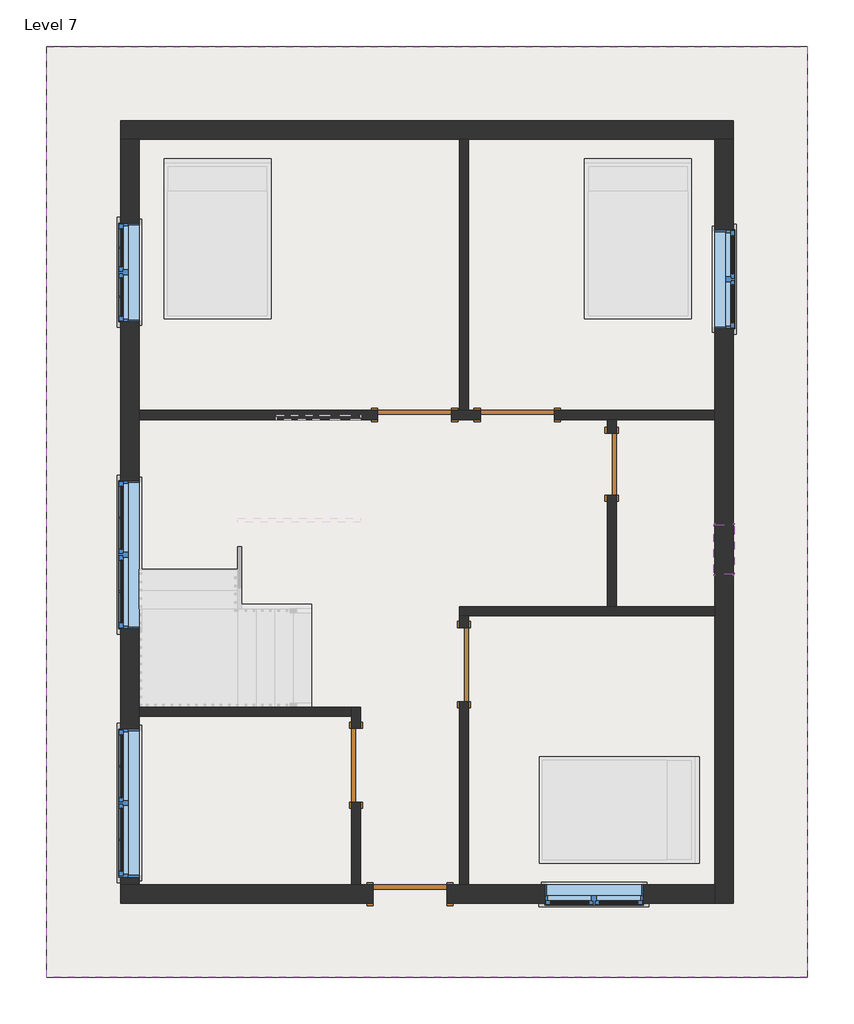
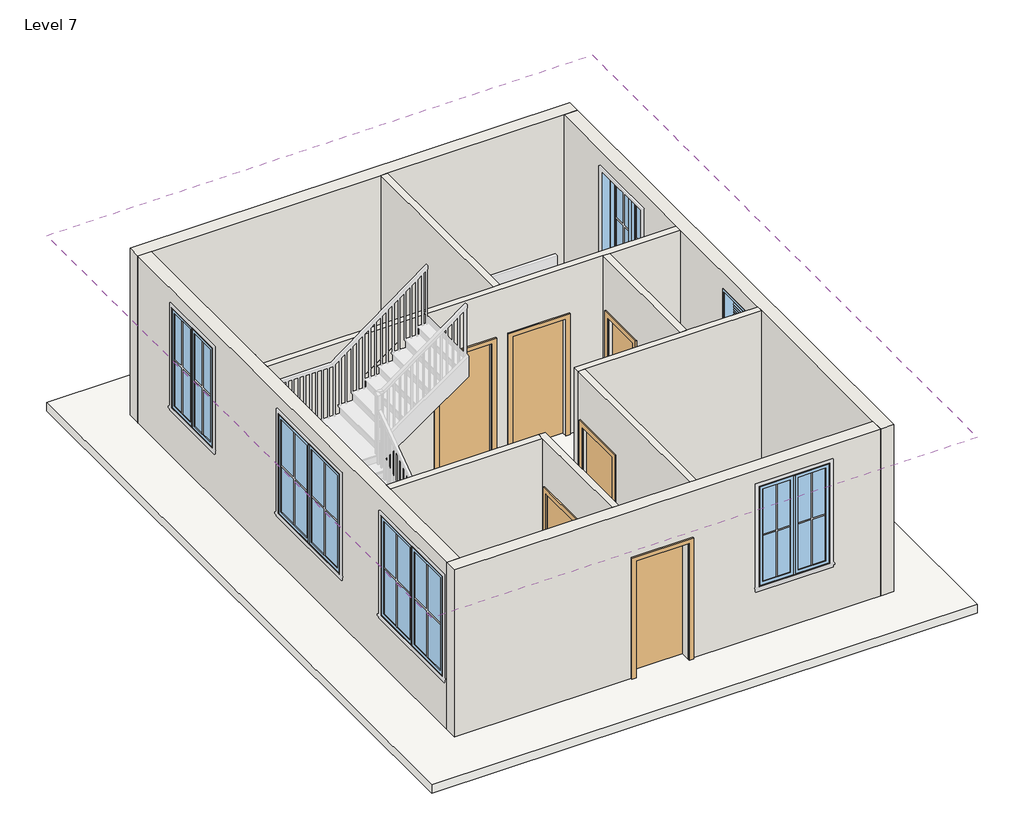
# One storey, part 1 of 3: 11 walls, 6 doors, 6 windows, 2 roofs.
"""IFC4 building model written with IfcOpenShell, lengths in millimetres."""

from ifc_helpers import new_model, si_unit, frame, origin, place, context, project, spatial, polyline, outline, extrude, faceted_brep, transform, mapped, element, save
from components import door_f2b275c1, single_flush_door_3_e5f9f3c4, single_flush_door_3_305aa2a5, single_flush_door_3_a90ba1ad, window_casement_double_win_4_6ca1769e, window_casement_double_win_6_ce442eab, window_f2d8fef0

model = new_model("IFC4")

# Units and contexts
model_context = context("Model", 3, world=origin())
ifc_project = project(units=[si_unit("LENGTHUNIT", "METRE", prefix="MILLI")], contexts=[model_context])

# Site, building, storey
site = spatial("IfcSite", under=ifc_project)
building = spatial("IfcBuilding", under=site)
storey = spatial("IfcBuildingStorey", under=building, Name="Level 7", Elevation=19050.0)

# Doors
placement = place(None, origin())
door_shape = door_f2b275c1(model_context)
element("IfcDoor", 1, ObjectType="Single-Flush : 2'6\"", at=placement, inside=storey, context=model_context, shape_type="MappedRepresentation", body=[
    mapped(door_shape, transform((1031.6394609, 262.5126239, 19050.0), x_axis=(0.0, 1.0, 0.0), y_axis=(-1.0, 0.0, 0.0), z_axis=(0.0, 0.0, 1.0))),
])
single_flush_door_3_shape = single_flush_door_3_e5f9f3c4(model_context)
element("IfcDoor", 2, ObjectType="Single-Flush : door 3'", at=placement, inside=storey, context=model_context, shape_type="MappedRepresentation", body=[
    mapped(single_flush_door_3_shape, transform((-1406.7605391, 872.1126239, 19050.0), x_axis=(1.0, 0.0, 0.0), y_axis=(0.0, 1.0, 0.0), z_axis=(0.0, 0.0, 1.0))),
])
element("IfcDoor", 3, ObjectType="Single-Flush : door 3'", at=placement, inside=storey, context=model_context, shape_type="MappedRepresentation", body=[
    mapped(single_flush_door_3_shape, transform((-2130.6605391, -3458.5873761, 19050.0), x_axis=(0.0, 1.0, 0.0), y_axis=(-1.0, 0.0, 0.0), z_axis=(0.0, 0.0, 1.0))),
])
single_flush_door_3_2_shape = single_flush_door_3_305aa2a5(model_context)
element("IfcDoor", 4, ObjectType="Single-Flush : door 3'", at=placement, inside=storey, context=model_context, shape_type="MappedRepresentation", body=[
    mapped(single_flush_door_3_2_shape, transform((-136.7605391, 872.1126239, 19050.0), x_axis=(-1.0, 0.0, 0.0), y_axis=(0.0, -1.0, 0.0), z_axis=(0.0, 0.0, 1.0))),
])
element("IfcDoor", 5, ObjectType="Single-Flush : door 3'", at=placement, inside=storey, context=model_context, shape_type="MappedRepresentation", body=[
    mapped(single_flush_door_3_2_shape, transform((-797.1605391, -2213.9873761, 19050.0), x_axis=(0.0, 1.0, 0.0), y_axis=(-1.0, 0.0, 0.0), z_axis=(0.0, 0.0, 1.0))),
])
single_flush_door_3_3_shape = single_flush_door_3_a90ba1ad(model_context)
element("IfcDoor", 6, ObjectType="Single-Flush : door 3'", at=placement, inside=storey, context=model_context, shape_type="MappedRepresentation", body=[
    mapped(single_flush_door_3_3_shape, transform((-1463.9105391, -5052.4373761, 19050.0), x_axis=(-1.0, 0.0, 0.0), y_axis=(0.0, -1.0, 0.0), z_axis=(0.0, 0.0, 1.0))),
])

# Roofs
element("IfcRoof", 7, ObjectType="Generic - 12\"", at=placement, inside=storey, context=model_context, shape_type="SweptSolid", body=[
    extrude(outline(polyline([(-5959.7105391, 5425.0626239), (3450.9894609, 5425.0626239), (3450.9894609, -6081.1373761), (-5959.7105391, -6081.1373761), (-5959.7105391, 5425.0626239)])), frame((0.0, 0.0, 18897.6), z_axis=(0.0, 0.0, 1.0), x_axis=(1.0, 0.0, 0.0)), (0.0, 0.0, 1.0), 152.4),
])
element("IfcRoof", 8, ObjectType="Generic - 12\"", at=placement, inside=storey, context=model_context, shape_type="SweptSolid", body=[
    extrude(outline(polyline([(-5959.7105391, 5425.0626239), (3450.9894609, 5425.0626239), (3450.9894609, -6081.1373761), (-5959.7105391, -6081.1373761), (-5959.7105391, 5425.0626239)])), frame((0.0, 0.0, 22098.0), z_axis=(0.0, 0.0, 1.0), x_axis=(1.0, 0.0, 0.0)), (0.0, 0.0, 1.0), 152.4),
])

# Walls
element("IfcWall", 9, ObjectType="WALL 4.5\"", at=placement, inside=storey, context=model_context, shape_type="SweptSolid", body=[
    extrude(outline(polyline([(-854.3105391, 929.2626239), (-854.3105391, 4282.0626239), (-740.0105391, 4282.0626239), (-740.0105391, 929.2626239), (-854.3105391, 929.2626239)])), frame((0.0, 0.0, 19050.0), z_axis=(0.0, 0.0, 1.0), x_axis=(1.0, 0.0, 0.0)), (0.0, 0.0, 1.0), 3048.0),
])
element("IfcWall", 10, ObjectType="WALL 4.5\"", at=placement, inside=storey, context=model_context, shape_type="Brep", body=[
    faceted_brep([(-949.5605391, 814.9626239, 19050.0), (-593.9605391, 814.9626239, 19050.0), (-593.9605391, 814.9626239, 21183.6), (320.4394609, 814.9626239, 21183.6), (320.4394609, 814.9626239, 19050.0), (974.4894609, 814.9626239, 19050.0), (1088.7894609, 814.9626239, 19050.0), (2307.9894609, 814.9626239, 19050.0), (2307.9894609, 814.9626239, 22098.0), (1088.7894609, 814.9626239, 22098.0), (974.4894609, 814.9626239, 22098.0), (-4816.7105391, 814.9626239, 22098.0), (-4816.7105391, 814.9626239, 19050.0), (-1863.9605391, 814.9626239, 19050.0), (-1863.9605391, 814.9626239, 21183.6), (-949.5605391, 814.9626239, 21183.6), (-593.9605391, 929.2626239, 21183.6), (-593.9605391, 929.2626239, 19050.0), (-740.0105391, 929.2626239, 19050.0), (-854.3105391, 929.2626239, 19050.0), (-949.5605391, 929.2626239, 19050.0), (-949.5605391, 929.2626239, 21183.6), (-1863.9605391, 929.2626239, 21183.6), (-1863.9605391, 929.2626239, 19050.0), (-4816.7105391, 929.2626239, 19050.0), (-4816.7105391, 929.2626239, 22098.0), (-854.3105391, 929.2626239, 22098.0), (-740.0105391, 929.2626239, 22098.0), (2307.9894609, 929.2626239, 22098.0), (2307.9894609, 929.2626239, 19050.0), (320.4394609, 929.2626239, 19050.0), (320.4394609, 929.2626239, 21183.6)], [[[0, 1, 2, 3, 4, 5, 6, 7, 8, 9, 10, 11, 12, 13, 14, 15]], [[16, 17, 18, 19, 20, 21, 22, 23, 24, 25, 26, 27, 28, 29, 30, 31]], [[13, 12, 24, 23]], [[30, 29, 7, 6, 5, 4]], [[20, 19, 18, 17, 1, 0]], [[8, 7, 29, 28]], [[12, 11, 25, 24]], [[21, 20, 0, 15]], [[22, 21, 15, 14]], [[23, 22, 14, 13]], [[2, 1, 17, 16]], [[3, 2, 16, 31]], [[4, 3, 31, 30]], [[11, 10, 9, 8, 28, 27, 26, 25]]]),
])
element("IfcWall", 11, ObjectType="WALL 4.5\"", at=placement, inside=storey, context=model_context, shape_type="SweptSolid", body=[
    extrude(outline(polyline([(814.9626239, 19050.0), (643.5126239, 19050.0), (643.5126239, 21082.0), (-118.4873761, 21082.0), (-118.4873761, 19050.0), (-1496.4373761, 19050.0), (-1496.4373761, 22098.0), (814.9626239, 22098.0), (814.9626239, 19050.0)])), frame((974.4894609, 0.0, 0.0), z_axis=(1.0, 0.0, 0.0), x_axis=(0.0, 1.0, 0.0)), (0.0, 0.0, 1.0), 114.3),
])
element("IfcWall", 12, ObjectType="WALL 4.5\"", at=placement, inside=storey, context=model_context, shape_type="Brep", body=[
    faceted_brep([(2307.9894609, -1496.4373761, 19050.0), (1088.7894609, -1496.4373761, 19050.0), (974.4894609, -1496.4373761, 19050.0), (-854.3105391, -1496.4373761, 19050.0), (-854.3105391, -1496.4373761, 22098.0), (974.4894609, -1496.4373761, 22098.0), (1088.7894609, -1496.4373761, 22098.0), (2307.9894609, -1496.4373761, 22098.0), (2307.9894609, -1610.7373761, 19050.0), (2307.9894609, -1610.7373761, 22098.0), (-740.0105391, -1610.7373761, 22098.0), (-854.3105391, -1610.7373761, 22098.0), (-854.3105391, -1610.7373761, 19050.0), (-740.0105391, -1610.7373761, 19050.0)], [[[0, 1, 2, 3, 4, 5, 6, 7]], [[8, 9, 10, 11, 12, 13]], [[3, 2, 1, 0, 8, 13, 12]], [[0, 7, 9, 8]], [[4, 3, 12, 11]], [[7, 6, 5, 4, 11, 10, 9]]]),
])
element("IfcWall", 13, ObjectType="WALL 4.5\"", at=placement, inside=storey, context=model_context, shape_type="SweptSolid", body=[
    extrude(outline(polyline([(-1610.7373761, 19050.0), (-1756.7873761, 19050.0), (-1756.7873761, 21183.6), (-2671.1873761, 21183.6), (-2671.1873761, 19050.0), (-4938.1373761, 19050.0), (-4938.1373761, 22098.0), (-1610.7373761, 22098.0), (-1610.7373761, 19050.0)])), frame((-854.3105391, 0.0, 0.0), z_axis=(1.0, 0.0, 0.0), x_axis=(0.0, 1.0, 0.0)), (0.0, 0.0, 1.0), 114.3),
])
element("IfcWall", 14, ObjectType="WALL 4.5\"", at=placement, inside=storey, context=model_context, shape_type="Brep", body=[
    faceted_brep([(-2073.5105391, -3001.3873761, 21183.6), (-2073.5105391, -3001.3873761, 19050.0), (-2073.5105391, -2741.0373761, 19050.0), (-2073.5105391, -2741.0373761, 22098.0), (-2073.5105391, -4938.1373761, 22098.0), (-2073.5105391, -4938.1373761, 19050.0), (-2073.5105391, -3915.7873761, 19050.0), (-2073.5105391, -3915.7873761, 21183.6), (-2187.8105391, -2741.0373761, 19050.0), (-2187.8105391, -2855.3373761, 19050.0), (-2187.8105391, -3001.3873761, 19050.0), (-2187.8105391, -3001.3873761, 21183.6), (-2187.8105391, -3915.7873761, 21183.6), (-2187.8105391, -3915.7873761, 19050.0), (-2187.8105391, -4938.1373761, 19050.0), (-2187.8105391, -4938.1373761, 22098.0), (-2187.8105391, -2855.3373761, 22098.0), (-2187.8105391, -2741.0373761, 22098.0)], [[[0, 1, 2, 3, 4, 5, 6, 7]], [[8, 9, 10, 11, 12, 13, 14, 15, 16, 17]], [[6, 5, 14, 13]], [[2, 1, 10, 9, 8]], [[5, 4, 15, 14]], [[3, 2, 8, 17]], [[11, 10, 1, 0]], [[12, 11, 0, 7]], [[13, 12, 7, 6]], [[4, 3, 17, 16, 15]]]),
])
element("IfcWall", 15, ObjectType="WALL 4.5\"", at=placement, inside=storey, context=model_context, shape_type="SweptSolid", body=[
    extrude(outline(polyline([(-4816.7105391, -2741.0373761), (-2187.8105391, -2741.0373761), (-2187.8105391, -2855.3373761), (-4816.7105391, -2855.3373761), (-4816.7105391, -2741.0373761)])), frame((0.0, 0.0, 19050.0), z_axis=(0.0, 0.0, 1.0), x_axis=(1.0, 0.0, 0.0)), (0.0, 0.0, 1.0), 3048.0),
])
element("IfcWall", 16, ObjectType="WALL 9\"", at=placement, inside=storey, context=model_context, shape_type="Brep", body=[
    faceted_brep([(-5045.3105391, 4282.0626239, 19050.0), (-4816.7105391, 4282.0626239, 19050.0), (-854.3105391, 4282.0626239, 19050.0), (-740.0105391, 4282.0626239, 19050.0), (2307.9894609, 4282.0626239, 19050.0), (2536.5894609, 4282.0626239, 19050.0), (2536.5894609, 4282.0626239, 22098.0), (2307.9894609, 4282.0626239, 22098.0), (-740.0105391, 4282.0626239, 22098.0), (-854.3105391, 4282.0626239, 22098.0), (-4816.7105391, 4282.0626239, 22098.0), (-5045.3105391, 4282.0626239, 22098.0), (-5045.3105391, 4510.6626239, 19050.0), (-5045.3105391, 4510.6626239, 22098.0), (2536.5894609, 4510.6626239, 22098.0), (2536.5894609, 4510.6626239, 19050.0)], [[[0, 1, 2, 3, 4, 5, 6, 7, 8, 9, 10, 11]], [[12, 13, 14, 15]], [[5, 4, 3, 2, 1, 0, 12, 15]], [[6, 5, 15, 14]], [[0, 11, 13, 12]], [[11, 10, 9, 8, 7, 6, 14, 13]]]),
])
element("IfcWall", 17, ObjectType="WALL 9\"", at=placement, inside=storey, context=model_context, shape_type="Brep", body=[
    faceted_brep([(2307.9894609, 4282.0626239, 19050.0), (2307.9894609, 929.2626239, 19050.0), (2307.9894609, 814.9626239, 19050.0), (2307.9894609, -1496.4373761, 19050.0), (2307.9894609, -1610.7373761, 19050.0), (2307.9894609, -4938.1373761, 19050.0), (2307.9894609, -5166.7373761, 19050.0), (2307.9894609, -5166.7373761, 22098.0), (2307.9894609, -4938.1373761, 22098.0), (2307.9894609, -1610.7373761, 22098.0), (2307.9894609, -1496.4373761, 22098.0), (2307.9894609, 814.9626239, 22098.0), (2307.9894609, 929.2626239, 22098.0), (2307.9894609, 4282.0626239, 22098.0), (2307.9894609, 1938.9126239, 21793.2), (2307.9894609, 1938.9126239, 19964.4), (2307.9894609, 3158.1126239, 19964.4), (2307.9894609, 3158.1126239, 21793.2), (2307.9894609, -486.7873761, 21793.2), (2307.9894609, -1096.3873761, 21793.2), (2307.9894609, -1096.3873761, 21183.6), (2307.9894609, -486.7873761, 21183.6), (2536.5894609, 4282.0626239, 19050.0), (2536.5894609, 4282.0626239, 22098.0), (2536.5894609, -5166.7373761, 22098.0), (2536.5894609, -5166.7373761, 19050.0), (2536.5894609, 1938.9126239, 21793.2), (2536.5894609, 3158.1126239, 21793.2), (2536.5894609, 3158.1126239, 19964.4), (2536.5894609, 1938.9126239, 19964.4), (2536.5894609, -486.7873761, 21793.2), (2536.5894609, -486.7873761, 21183.6), (2536.5894609, -1096.3873761, 21183.6), (2536.5894609, -1096.3873761, 21793.2)], [[[0, 1, 2, 3, 4, 5, 6, 7, 8, 9, 10, 11, 12, 13], [14, 15, 16, 17], [18, 19, 20, 21]], [[22, 23, 24, 25], [26, 27, 28, 29], [30, 31, 32, 33]], [[6, 5, 4, 3, 2, 1, 0, 22, 25]], [[0, 13, 23, 22]], [[7, 6, 25, 24]], [[15, 14, 26, 29]], [[16, 15, 29, 28]], [[17, 16, 28, 27]], [[14, 17, 27, 26]], [[31, 30, 18, 21]], [[32, 31, 21, 20]], [[33, 32, 20, 19]], [[30, 33, 19, 18]], [[13, 12, 11, 10, 9, 8, 7, 24, 23]]]),
])
element("IfcWall", 18, ObjectType="WALL 9\"", at=placement, inside=storey, context=model_context, shape_type="Brep", body=[
    faceted_brep([(-1921.1105391, -4938.1373761, 21183.6), (-1921.1105391, -4938.1373761, 19050.0), (-2073.5105391, -4938.1373761, 19050.0), (-2187.8105391, -4938.1373761, 19050.0), (-4816.7105391, -4938.1373761, 19050.0), (-5045.3105391, -4938.1373761, 19050.0), (-5045.3105391, -4938.1373761, 22098.0), (-4816.7105391, -4938.1373761, 22098.0), (-2187.8105391, -4938.1373761, 22098.0), (-2073.5105391, -4938.1373761, 22098.0), (-854.3105391, -4938.1373761, 22098.0), (-740.0105391, -4938.1373761, 22098.0), (2307.9894609, -4938.1373761, 22098.0), (2307.9894609, -4938.1373761, 19050.0), (-740.0105391, -4938.1373761, 19050.0), (-854.3105391, -4938.1373761, 19050.0), (-1006.7105391, -4938.1373761, 19050.0), (-1006.7105391, -4938.1373761, 21183.6), (202.9644609, -4938.1373761, 21793.2), (202.9644609, -4938.1373761, 19964.4), (1422.1644609, -4938.1373761, 19964.4), (1422.1644609, -4938.1373761, 21793.2), (-5045.3105391, -5166.7373761, 19050.0), (-1921.1105391, -5166.7373761, 19050.0), (-1921.1105391, -5166.7373761, 21183.6), (-1006.7105391, -5166.7373761, 21183.6), (-1006.7105391, -5166.7373761, 19050.0), (2307.9894609, -5166.7373761, 19050.0), (2307.9894609, -5166.7373761, 22098.0), (-5045.3105391, -5166.7373761, 22098.0), (202.9644609, -5166.7373761, 21793.2), (1422.1644609, -5166.7373761, 21793.2), (1422.1644609, -5166.7373761, 19964.4), (202.9644609, -5166.7373761, 19964.4)], [[[0, 1, 2, 3, 4, 5, 6, 7, 8, 9, 10, 11, 12, 13, 14, 15, 16, 17], [18, 19, 20, 21]], [[22, 23, 24, 25, 26, 27, 28, 29], [30, 31, 32, 33]], [[5, 4, 3, 2, 1, 23, 22]], [[16, 15, 14, 13, 27, 26]], [[13, 12, 28, 27]], [[6, 5, 22, 29]], [[19, 18, 30, 33]], [[20, 19, 33, 32]], [[21, 20, 32, 31]], [[18, 21, 31, 30]], [[24, 23, 1, 0]], [[25, 24, 0, 17]], [[26, 25, 17, 16]], [[12, 11, 10, 9, 8, 7, 6, 29, 28]]]),
])
element("IfcWall", 19, ObjectType="WALL 9\"", at=placement, inside=storey, context=model_context, shape_type="Brep", body=[
    faceted_brep([(-4816.7105391, -4938.1373761, 19050.0), (-4816.7105391, -2855.3373761, 19050.0), (-4816.7105391, -2741.0373761, 19050.0), (-4816.7105391, 814.9626239, 19050.0), (-4816.7105391, 929.2626239, 19050.0), (-4816.7105391, 4282.0626239, 19050.0), (-4816.7105391, 4282.0626239, 22098.0), (-4816.7105391, 929.2626239, 22098.0), (-4816.7105391, 814.9626239, 22098.0), (-4816.7105391, -2741.0373761, 22098.0), (-4816.7105391, -2855.3373761, 22098.0), (-4816.7105391, -4938.1373761, 22098.0), (-4816.7105391, -3010.9123761, 21793.2), (-4816.7105391, -3010.9123761, 19964.4), (-4816.7105391, -4839.7123761, 19964.4), (-4816.7105391, -4839.7123761, 21793.2), (-4816.7105391, 59.3126239, 21793.2), (-4816.7105391, 59.3126239, 19964.4), (-4816.7105391, -1769.4873761, 19964.4), (-4816.7105391, -1769.4873761, 21793.2), (-4816.7105391, 3243.8376239, 21793.2), (-4816.7105391, 3243.8376239, 19964.4), (-4816.7105391, 2024.6376239, 19964.4), (-4816.7105391, 2024.6376239, 21793.2), (-5045.3105391, -4938.1373761, 19050.0), (-5045.3105391, -4938.1373761, 22098.0), (-5045.3105391, 4282.0626239, 22098.0), (-5045.3105391, 4282.0626239, 19050.0), (-5045.3105391, -3010.9123761, 21793.2), (-5045.3105391, -4839.7123761, 21793.2), (-5045.3105391, -4839.7123761, 19964.4), (-5045.3105391, -3010.9123761, 19964.4), (-5045.3105391, 59.3126239, 21793.2), (-5045.3105391, -1769.4873761, 21793.2), (-5045.3105391, -1769.4873761, 19964.4), (-5045.3105391, 59.3126239, 19964.4), (-5045.3105391, 3243.8376239, 21793.2), (-5045.3105391, 2024.6376239, 21793.2), (-5045.3105391, 2024.6376239, 19964.4), (-5045.3105391, 3243.8376239, 19964.4)], [[[0, 1, 2, 3, 4, 5, 6, 7, 8, 9, 10, 11], [12, 13, 14, 15], [16, 17, 18, 19], [20, 21, 22, 23]], [[24, 25, 26, 27], [28, 29, 30, 31], [32, 33, 34, 35], [36, 37, 38, 39]], [[5, 4, 3, 2, 1, 0, 24, 27]], [[6, 5, 27, 26]], [[0, 11, 25, 24]], [[13, 12, 28, 31]], [[14, 13, 31, 30]], [[15, 14, 30, 29]], [[12, 15, 29, 28]], [[17, 16, 32, 35]], [[18, 17, 35, 34]], [[19, 18, 34, 33]], [[16, 19, 33, 32]], [[21, 20, 36, 39]], [[22, 21, 39, 38]], [[23, 22, 38, 37]], [[20, 23, 37, 36]], [[11, 10, 9, 8, 7, 6, 26, 25]]]),
])

# Windows
window_casement_double_win_4_shape = window_casement_double_win_4_6ca1769e(model_context)
element("IfcWindow", 20, ObjectType="Window-Casement-Double : win 4'", at=placement, inside=storey, context=model_context, shape_type="MappedRepresentation", body=[
    mapped(window_casement_double_win_4_shape, transform((812.5644609, -5052.4373761, 19050.0), x_axis=(-1.0, 0.0, 0.0), y_axis=(0.0, -1.0, 0.0), z_axis=(0.0, 0.0, 1.0))),
])
element("IfcWindow", 21, ObjectType="Window-Casement-Double : win 4'", at=placement, inside=storey, context=model_context, shape_type="MappedRepresentation", body=[
    mapped(window_casement_double_win_4_shape, transform((2422.2894609, 2548.5126239, 19050.0), x_axis=(0.0, -1.0, 0.0), y_axis=(1.0, 0.0, 0.0), z_axis=(0.0, 0.0, 1.0))),
])
element("IfcWindow", 22, ObjectType="Window-Casement-Double : win 4'", at=placement, inside=storey, context=model_context, shape_type="MappedRepresentation", body=[
    mapped(window_casement_double_win_4_shape, transform((-4931.0105391, 2634.2376239, 19050.0), x_axis=(0.0, 1.0, 0.0), y_axis=(-1.0, 0.0, 0.0), z_axis=(0.0, 0.0, 1.0))),
])
window_casement_double_win_6_shape = window_casement_double_win_6_ce442eab(model_context)
element("IfcWindow", 23, ObjectType="Window-Casement-Double : win 6'", at=placement, inside=storey, context=model_context, shape_type="MappedRepresentation", body=[
    mapped(window_casement_double_win_6_shape, transform((-4931.0105391, -3925.3123761, 19050.0), x_axis=(0.0, 1.0, 0.0), y_axis=(-1.0, 0.0, 0.0), z_axis=(0.0, 0.0, 1.0))),
])
element("IfcWindow", 24, ObjectType="Window-Casement-Double : win 6'", at=placement, inside=storey, context=model_context, shape_type="MappedRepresentation", body=[
    mapped(window_casement_double_win_6_shape, transform((-4931.0105391, -855.0873761, 19050.0), x_axis=(0.0, 1.0, 0.0), y_axis=(-1.0, 0.0, 0.0), z_axis=(0.0, 0.0, 1.0))),
])
window_shape = window_f2d8fef0(model_context)
element("IfcWindow", 25, ObjectType="Window-Louvers : 24\" x 24\"", at=placement, inside=storey, context=model_context, shape_type="MappedRepresentation", body=[
    mapped(window_shape, transform((2428.6394609, -791.5873761, 20269.2), x_axis=(0.0, -1.0, 0.0), y_axis=(1.0, 0.0, 0.0), z_axis=(0.0, 0.0, 1.0))),
])

save(model, "model.ifc")

# Revit data of these elements
# Type "Single-Flush : 2'6\""
#   Type Mark = "9"
#   Construction Type Id = "MDOOR"
#   Assembly Code = "C1020"
#   Analytic Construction = "Metal"
#   Thickness = 0' - 2"
#   Heat Transfer Coefficient (U) = 0.651978 BTU/(h·ft²·°F)
#   Height = 6' - 8"
#   Trim Projection Ext = 0' - 1"
#   Trim Projection Int = 0' - 1"
#   Trim Width = 0' - 3"
#   Width = 2' - 6"
#   Define Thermal Properties by = 1
#   Door Material = Door - Panel
#   Frame Material = Door - Frame
#   Visual Light Transmittance = 0
#   Solar Heat Gain Coefficient = 0
#   Function = (empty or 0)
#   Wall Closure = (empty or 0)
# Type "Single-Flush : door 3'"
#   Type Mark = "8"
#   Construction Type Id = "MDOOR"
#   Assembly Code = "C1020"
#   Analytic Construction = "Metal"
#   Thickness = 0' - 2"
#   Heat Transfer Coefficient (U) = 0.651978 BTU/(h·ft²·°F)
#   Height = 7' - 0"
#   Trim Projection Ext = 0' - 1"
#   Trim Projection Int = 0' - 1"
#   Trim Width = 0' - 3"
#   Width = 3' - 0"
#   Define Thermal Properties by = 1
#   Door Material = Door - Panel
#   Frame Material = Door - Frame
#   Visual Light Transmittance = 0
#   Solar Heat Gain Coefficient = 0
#   Function = (empty or 0)
#   Wall Closure = (empty or 0)
# Type "Generic - 12\""
#   Assembly Code = "B1020"
#   Layers, outside or top first: 0' - 6" no material (function 1)
# Type "WALL 4.5\""
#   Assembly Code = "B2010"
#   Layers, outside or top first: 0' - 4 1/2" no material (function 1)
# Type "WALL 9\""
#   Assembly Code = "B2010"
#   Layers, outside or top first: 0' - 9" no material (function 1)
# Type "Window-Casement-Double : win 4'"
#   Type Mark = "19"
#   Fire Rating = "0.5h"
#   Assembly Code = "B2020100"
#   Analytic Construction = "Double glazing - domestic"
#   Frame Extension [instance default] = 0' - 0 1/4"
#   Window Inset [instance default] = 0' - 0"
#   Wall Thickness [instance default] = 0' - 6"
#   Interior Wall Closure [instance default] = 0' - 2 1/4"
#   Half Width = 2' - 0"
#   Visual Light Transmittance = 0.81
#   Thermal Resistance (R) = 1.8146 (h·ft²·°F)/BTU
#   Solar Heat Gain Coefficient = 0.76
#   Rough Width = 4' - 0 1/2"
#   Rough Height = 6' - 0 1/2"
#   Height = 6' - 0"
#   Heat Transfer Coefficient (U) = 0.5511 BTU/(h·ft²·°F)
#   Exterior Wall Closure [instance default] = 0' - 1 1/4"
#   Extension Jamb [instance default] = 0' - 2 1/4"
#   Default Sill Height = 3' - 0"
#   Width = 4' - 0"
#   Muntin Visibility = yes
#   Interior Trim Visibility [instance default] = yes
#   Exterior Trim Visibility [instance default] = yes
#   Extension Jamb Visibility [instance default] = yes
#   Interior Trim Material = Wood - Stained
#   Muntin Pattern = Muntin Pattern_2x2 : Muntin Pattern_2x2
#   Interior Trim = Trim-Window-Interior-Flat : Picture Frame
#   Interior Frame Material = Wood - Stained
#   Glass Panel Material = Glass
#   Exterior Trim Material = Clad - White
#   Exterior Trim = Trim-Window-Exterior-Flat : with Sill
#   Exterior Frame Material = Clad - White
#   Wall Closure = (empty or 0)
# Type "Window-Casement-Double : win 6'"
#   Type Mark = "18"
#   Fire Rating = "0.5h"
#   Assembly Code = "B2020100"
#   Analytic Construction = "Double glazing - domestic"
#   Frame Extension [instance default] = 0' - 0 1/4"
#   Window Inset [instance default] = 0' - 0"
#   Wall Thickness [instance default] = 0' - 6"
#   Interior Wall Closure [instance default] = 0' - 2 1/4"
#   Half Width = 3' - 0"
#   Visual Light Transmittance = 0.81
#   Thermal Resistance (R) = 1.8146 (h·ft²·°F)/BTU
#   Solar Heat Gain Coefficient = 0.76
#   Rough Width = 6' - 0 1/2"
#   Rough Height = 6' - 0 1/2"
#   Height = 6' - 0"
#   Heat Transfer Coefficient (U) = 0.5511 BTU/(h·ft²·°F)
#   Exterior Wall Closure [instance default] = 0' - 1 1/4"
#   Extension Jamb [instance default] = 0' - 2 1/4"
#   Default Sill Height = 3' - 0"
#   Width = 6' - 0"
#   Muntin Visibility = yes
#   Interior Trim Visibility [instance default] = yes
#   Exterior Trim Visibility [instance default] = yes
#   Extension Jamb Visibility [instance default] = yes
#   Interior Trim Material = Wood - Stained
#   Muntin Pattern = Muntin Pattern_2x2 : Muntin Pattern_2x2
#   Interior Trim = Trim-Window-Interior-Flat : Picture Frame
#   Interior Frame Material = Wood - Stained
#   Glass Panel Material = Glass
#   Exterior Trim Material = Clad - White
#   Exterior Trim = Trim-Window-Exterior-Flat : with Sill
#   Exterior Frame Material = Clad - White
#   Wall Closure = (empty or 0)
# Type "Window-Louvers : 24\" x 24\""
#   Type Mark = "20"
#   Construction Type Id = "GSP4R"
#   Assembly Code = "B20"
#   Analytic Construction = "1/8 in Pilkington single glazing"
#   Visual Light Transmittance = 0.9
#   Thermal Resistance (R) = 1.53941 (h·ft²·°F)/BTU
#   Solar Heat Gain Coefficient = 0.78
#   Max Height = 1' - 11.74264"
#   Height = 2' - 0"
#   Heat Transfer Coefficient (U) = 0.6496 BTU/(h·ft²·°F)
#   Blade Width [instance default] = 1' - 10 1/2"
#   Blade Vertical Thickness = 0' - 0.35355"
#   Blade Thickness = 0' - 0 1/4"
#   Blade Spacing = 0' - 1 1/2"
#   Blade Height = 0' - 1.85355"
#   Blade Depth = 0' - 3"
#   Blade Angle = 45.00°
#   Default Sill Height = 3' - 0"
#   Trim Projection_Exterior = 0' - 0 1/2"
#   Trim Projection_Interior = 0' - 0 1/2"
#   Trim Width_Exterior = 0' - 1 1/2"
#   Trim Width_Interior = 0' - 1 1/2"
#   Width = 2' - 0"
#   Max Blade Count = 12
#   Define Thermal Properties by = 1
#   Blade Count = 12
#   Frame Material = Birch
#   Louver Material = Birch
#   Trim Exterior Material = Birch
#   Trim Interior Material = Birch
#   Wall Closure = (empty or 0)
# Element 1 (IfcDoor, "Single-Flush : 2'6\"")
#   Phase Created = New Construction
#   Materials on its faces: "Door - Frame", "Door - Panel"
# Elements 2, 3, 4, 5, 6 (IfcDoor, "Single-Flush : door 3'")
#   Phase Created = New Construction
#   Materials on its faces: "Door - Frame", "Door - Panel"
# Element 7 (IfcRoof, "Generic - 12\"")
#   built-in parameter 1001705 = 62.5 (stored number, unit not read)
#   built-in parameter 1001701 = -0.5 (stored number, unit not read)
#   built-in parameter 1001710 = 33615
#   Phase Created = New Construction
#   Materials on its faces: "Wood Planks", "Wood - Stained"
# Element 8 (IfcRoof, "Generic - 12\"")
#   built-in parameter 1001705 = 73 (stored number, unit not read)
#   built-in parameter 1001701 = 10 (stored number, unit not read)
#   built-in parameter 1001710 = 33615
#   Phase Created = New Construction
#   Materials on its faces: "Wood Planks", "Wood - Stained"
# Elements 9, 10, 11, 12, 13, 14, 15 (IfcWall, "WALL 4.5\"")
#   Top Offset = 0' - 0"
#   Base Offset = 0' - 0"
#   Unconnected Height = 10' - 0"
#   wall height = 10' - 0"
#   Phase Created = New Construction
#   Base Constraint = Level 7
#   Materials on its faces: "Default Wall"
# Elements 16, 17, 18, 19 (IfcWall, "WALL 9\"")
#   Top Offset = 0' - 0"
#   Base Offset = 0' - 0"
#   Unconnected Height = 10' - 0"
#   wall height = 10' - 0"
#   Phase Created = New Construction
#   Base Constraint = Level 7
#   Materials on its faces: "Default Wall", "Door - Frame"
# Element 20 (IfcWindow, "Window-Casement-Double : win 4'")
#   Mark = "39"
#   Window Inset = 0' - 0"
#   Interior Wall Closure = 0' - 2 1/4"
#   Frame Extension = 0' - 0 1/4"
#   Exterior Wall Closure = 0' - 1 1/4"
#   Interior Trim Visibility = yes
#   Exterior Trim Visibility = yes
#   Phase Created = New Construction
#   Materials on its faces: "Wood - Stained", "Glass", "Clad - White"
# Element 21 (IfcWindow, "Window-Casement-Double : win 4'")
#   Mark = "40"
#   Window Inset = 0' - 0"
#   Interior Wall Closure = 0' - 2 1/4"
#   Frame Extension = 0' - 0 1/4"
#   Exterior Wall Closure = 0' - 1 1/4"
#   Interior Trim Visibility = yes
#   Exterior Trim Visibility = yes
#   Phase Created = New Construction
#   Materials on its faces: "Wood - Stained", "Glass", "Clad - White"
# Element 22 (IfcWindow, "Window-Casement-Double : win 4'")
#   Mark = "41"
#   Window Inset = 0' - 0"
#   Interior Wall Closure = 0' - 2 1/4"
#   Frame Extension = 0' - 0 1/4"
#   Exterior Wall Closure = 0' - 1 1/4"
#   Interior Trim Visibility = yes
#   Exterior Trim Visibility = yes
#   Phase Created = New Construction
#   Materials on its faces: "Wood - Stained", "Glass", "Clad - White"
# Element 23 (IfcWindow, "Window-Casement-Double : win 6'")
#   Mark = "37"
#   Window Inset = 0' - 0"
#   Interior Wall Closure = 0' - 2 1/4"
#   Frame Extension = 0' - 0 1/4"
#   Exterior Wall Closure = 0' - 1 1/4"
#   Interior Trim Visibility = yes
#   Exterior Trim Visibility = yes
#   Phase Created = New Construction
#   Materials on its faces: "Wood - Stained", "Glass", "Clad - White"
# Element 24 (IfcWindow, "Window-Casement-Double : win 6'")
#   Mark = "38"
#   Window Inset = 0' - 0"
#   Interior Wall Closure = 0' - 2 1/4"
#   Frame Extension = 0' - 0 1/4"
#   Exterior Wall Closure = 0' - 1 1/4"
#   Interior Trim Visibility = yes
#   Exterior Trim Visibility = yes
#   Phase Created = New Construction
#   Materials on its faces: "Wood - Stained", "Glass", "Clad - White"
# Element 25 (IfcWindow, "Window-Louvers : 24\" x 24\"")
#   Mark = "42"
#   Blade Width = 1' - 10 1/2"
#   Phase Created = New Construction
#   Materials on its faces: "Birch"
# Materials
#   "Door - Panel": class "Wood", colour RGB 210 159 95, transparency 0, Cost = 0
#   "Door - Frame": colour RGB 118 70 51, transparency 0, Cost = 0
#   "Wood - Stained": class "Wood", colour RGB 224 178 126, transparency 0, Cost = 0
#   "Glass": class "Glass", colour RGB 0 128 192, transparency 0.75, Description = "Soda Lime Glass", Cost = 0
#   "Clad - White": class "Wood", colour RGB 242 242 238, transparency 0, Cost = 0
#   "Birch": class "Wood", colour RGB 224 178 126, transparency 0, Description = "Betula Alleghaniensis", Cost = 0
#   "Wood Planks": class "Wood", colour RGB 193 160 115, transparency 0, Description = "Physical material.", Cost = 0
#   "Default Wall": colour RGB 128 128 128, transparency 0, Cost = 0
